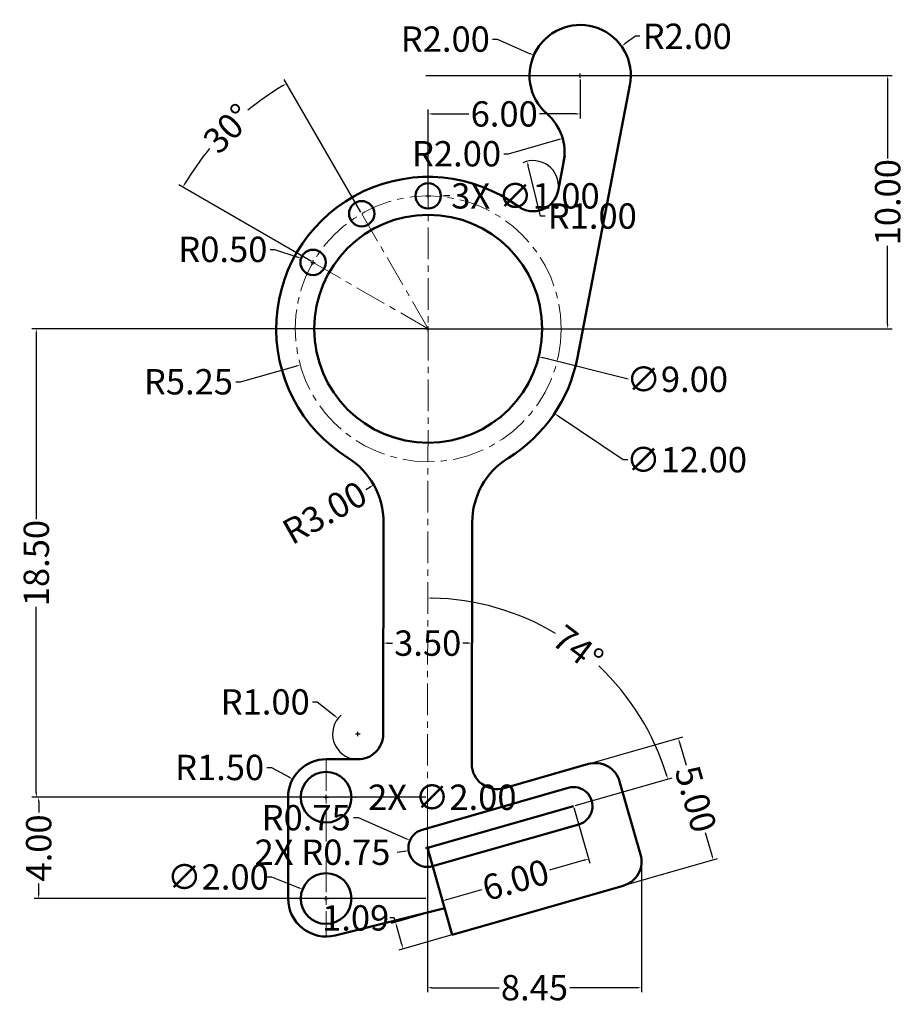
# Model space of a CAD drawing. Units: inches. Extents: x 11.4 to 46.3, y -1.7 to 37.2.
import ezdxf

# ---------------------------------------------------------------- set-up
doc = ezdxf.new("R2010")
doc.units = ezdxf.units.IN
doc.header["$MEASUREMENT"] = 0
doc.linetypes.add('CENTER', pattern=[2, 1.25, -0.25, 0.25, -0.25])
for name, color, linetype, lineweight in [('M-CNTR', 1, 'CENTER', 18), ('M-CONS', 8, 'Continuous', 13), ('M-DIMS', 2, 'Continuous', 25), ('M-OUTL', 7, 'Continuous', 50)]:
    doc.layers.add(name, color=color, linetype=linetype, lineweight=lineweight)
doc.styles.get("Standard").update_dxf_attribs({"font": 'arial.ttf'})
doc.dimstyles.get("Standard").update_dxf_attribs({"dimtxt": 1, "dimasz": 0.18, "dimexe": 0.18, "dimexo": 0.0625, "dimgap": 0.09, "dimtad": 0, "dimtoh": 1, "dimzin": 0, "dimdsep": 46, "dimtxsty": 'Standard', "dimcen": 0.09, "dimadec": 0, "dimazin": 0, "dimtfac": 1, "dimtofl": 0, "dimtmove": 0, "dimatfit": 3, "dimfxl": 1, "dimtolj": 1, "dimtzin": 0, "dimarcsym": 0})

# ---------------------------------------------------------------- blocks, each defined once
blk = doc.blocks.new('*D1')
at = {"layer": 'Defpoints', "color": 0, "transparency": 16777216}
for p in [(32.154, 7.358), (38.748, 4.047), (33.532, 2.552)]:
    blk.add_point(p, dxfattribs=at)
at = {"layer": 'M-DIMS', "color": 0, "lineweight": -2, "transparency": 16777216}
for p, q in [((32.214, 7.375), (37.543, 8.903)), ((37.42, 8.681), (37.677, 7.784)), ((38.699, 4.22), (38.442, 5.117)), ((33.592, 2.569), (38.921, 4.097))]:
    blk.add_line(p, q, dxfattribs=at)
at = {"layer": 'M-DIMS', "color": 0, "transparency": 16777216}
for points in [[(37.449, 8.689), (37.391, 8.672), (37.37, 8.854)], [(38.728, 4.229), (38.67, 4.212), (38.748, 4.047)]]:
    blk.add_solid(points, dxfattribs=at)
at = {"layer": 'M-DIMS', "color": 0, "transparency": 16777216, "insert": (38.059, 6.45), "char_height": 1, "attachment_point": 5, "rotation": 286}
blk.add_mtext('\\A1;5.00', dxfattribs=at)
blk = doc.blocks.new('*D2')
at = {"layer": 'Defpoints', "color": 0, "transparency": 16777216}
for p in [(33.232, 6.172), (27.464, 4.518), (33.83, 4.085)]:
    blk.add_point(p, dxfattribs=at)
at = {"layer": 'M-DIMS', "color": 0, "lineweight": -2, "transparency": 16777216}
for p, q in [((33.249, 6.112), (33.88, 3.912)), ((27.481, 4.458), (28.112, 2.258)), ((33.657, 4.035), (32.282, 3.641)), ((28.236, 2.48), (29.61, 2.875))]:
    blk.add_line(p, q, dxfattribs=at)
at = {"layer": 'M-DIMS', "color": 0, "transparency": 16777216}
for points in [[(33.649, 4.064), (33.665, 4.006), (33.83, 4.085)], [(28.227, 2.509), (28.244, 2.452), (28.063, 2.431)]]:
    blk.add_solid(points, dxfattribs=at)
at = {"layer": 'M-DIMS', "color": 0, "transparency": 16777216, "insert": (30.946, 3.258), "char_height": 1, "attachment_point": 5, "rotation": 16}
blk.add_mtext('\\A1;6.00', dxfattribs=at)
blk = doc.blocks.new('*D3')
at = {"layer": 'Defpoints', "color": 0, "transparency": 16777216}
for p in [(27.495, 25.018), (34.951, 10.945), (27.464, 6.518), (33.232, 6.172), (27.464, 4.518)]:
    blk.add_point(p, dxfattribs=at)
at = {"layer": 'M-DIMS', "color": 0, "lineweight": -2, "transparency": 16777216}
blk.add_line((33.292, 6.189), (37.122, 7.287), dxfattribs=at)
for start, end in [(59.1572, 88.8599), (17.0449, 46.7476)]:
    blk.add_arc((27.461, 4.517), 9.87, start, end, dxfattribs=at)
at = {"layer": 'M-DIMS', "color": 0, "transparency": 16777216}
for points in [[(27.657, 14.355), (27.658, 14.415), (27.477, 14.387)], [(36.926, 7.419), (36.869, 7.402), (36.949, 7.238)]]:
    blk.add_solid(points, dxfattribs=at)
at = {"layer": 'M-DIMS', "color": 0, "transparency": 16777216, "insert": (33.408, 12.395), "char_height": 1, "attachment_point": 5, "rotation": 322.9524}
blk.add_mtext('\\A1;74°', dxfattribs=at)
blk = doc.blocks.new('*D4')
at = {"layer": 'Defpoints', "color": 0, "transparency": 16777216}
for p in [(23.932, 9.637), (24.718, 9.019)]:
    blk.add_point(p, dxfattribs=at)
at = {"layer": 'M-DIMS', "color": 0, "lineweight": -2, "transparency": 16777216}
for p, q in [((22.926, 10.286), (23.106, 10.286)), ((23.106, 10.286), (23.791, 9.748)), ((24.628, 9.019), (24.808, 9.019)), ((24.718, 8.929), (24.718, 9.109))]:
    blk.add_line(p, q, dxfattribs=at)
blk.add_arc((24.718, 9.019), 1, 131.5148, 266.3238, dxfattribs=at)
at = {"layer": 'M-DIMS', "color": 0, "transparency": 16777216}
blk.add_solid([(23.809, 9.772), (23.772, 9.724), (23.932, 9.637)], dxfattribs=at)
at = {"layer": 'M-DIMS', "color": 0, "transparency": 16777216, "insert": (21.061, 10.286), "char_height": 1, "attachment_point": 5}
blk.add_mtext('\\A1;R1.00', dxfattribs=at)
blk = doc.blocks.new('*D5')
at = {"layer": 'Defpoints', "color": 0, "transparency": 16777216}
for p in [(26.777, 4.819), (27.464, 4.518)]:
    blk.add_point(p, dxfattribs=at)
at = {"layer": 'M-DIMS', "color": 0, "lineweight": -2, "transparency": 16777216}
for p, q in [((24.55, 5.715), (24.73, 5.715)), ((24.73, 5.715), (26.612, 4.891)), ((27.374, 4.518), (27.554, 4.518)), ((27.464, 4.428), (27.464, 4.608))]:
    blk.add_line(p, q, dxfattribs=at)
at = {"layer": 'M-DIMS', "color": 0, "transparency": 16777216}
blk.add_solid([(26.624, 4.918), (26.6, 4.863), (26.777, 4.819)], dxfattribs=at)
at = {"layer": 'M-DIMS', "color": 0, "transparency": 16777216, "insert": (22.679, 5.715), "char_height": 1, "attachment_point": 5}
blk.add_mtext('\\A1;R0.75', dxfattribs=at)
blk = doc.blocks.new('*D6')
at = {"layer": 'Defpoints', "color": 0, "transparency": 16777216}
for p in [(22.475, 27.803), (22.948, 27.643)]:
    blk.add_point(p, dxfattribs=at)
at = {"layer": 'M-DIMS', "color": 0, "lineweight": -2, "transparency": 16777216}
for p, q in [((21.254, 28.154), (21.434, 28.154)), ((21.434, 28.154), (22.304, 27.86)), ((22.858, 27.643), (23.038, 27.643)), ((22.948, 27.553), (22.948, 27.733))]:
    blk.add_line(p, q, dxfattribs=at)
at = {"layer": 'M-DIMS', "color": 0, "transparency": 16777216}
blk.add_solid([(22.314, 27.889), (22.294, 27.832), (22.475, 27.803)], dxfattribs=at)
at = {"layer": 'M-DIMS', "color": 0, "transparency": 16777216, "insert": (19.388, 28.154), "char_height": 1, "attachment_point": 5}
blk.add_mtext('\\A1;R0.50', dxfattribs=at)
blk = doc.blocks.new('*D7')
at = {"layer": 'Defpoints', "color": 0, "transparency": 16777216}
for p in [(31.664, 35.821), (33.495, 35.016)]:
    blk.add_point(p, dxfattribs=at)
at = {"layer": 'M-DIMS', "color": 0, "lineweight": -2, "transparency": 16777216}
for p, q in [((30.037, 36.458), (30.217, 36.458)), ((30.217, 36.458), (31.499, 35.894)), ((33.405, 35.016), (33.585, 35.016)), ((33.495, 34.926), (33.495, 35.106))]:
    blk.add_line(p, q, dxfattribs=at)
at = {"layer": 'M-DIMS', "color": 0, "transparency": 16777216}
blk.add_solid([(31.511, 35.921), (31.487, 35.866), (31.664, 35.821)], dxfattribs=at)
at = {"layer": 'M-DIMS', "color": 0, "transparency": 16777216, "insert": (28.171, 36.458), "char_height": 1, "attachment_point": 5}
blk.add_mtext('\\A1;R2.00', dxfattribs=at)
blk = doc.blocks.new('*D8')
at = {"layer": 'Defpoints', "color": 0, "transparency": 16777216}
for p in [(31.402, 31.633), (31.637, 30.661)]:
    blk.add_point(p, dxfattribs=at)
at = {"layer": 'M-DIMS', "color": 0, "lineweight": -2, "transparency": 16777216}
for p, q in [((31.926, 29.47), (31.444, 31.458)), ((32.106, 29.47), (31.926, 29.47))]:
    blk.add_line(p, q, dxfattribs=at)
blk.add_arc((31.637, 30.661), 1, 352.6761, 113.9298, dxfattribs=at)
at = {"layer": 'M-DIMS', "color": 0, "transparency": 16777216}
blk.add_solid([(31.473, 31.465), (31.415, 31.451), (31.402, 31.633)], dxfattribs=at)
at = {"layer": 'M-DIMS', "color": 0, "transparency": 16777216, "insert": (33.971, 29.47), "char_height": 1, "attachment_point": 5}
blk.add_mtext('\\A1;R1.00', dxfattribs=at)
blk = doc.blocks.new('*D9')
at = {"layer": 'Defpoints', "color": 0, "transparency": 16777216}
for p in [(35.124, 36.176), (33.495, 35.016)]:
    blk.add_point(p, dxfattribs=at)
at = {"layer": 'M-DIMS', "color": 0, "lineweight": -2, "transparency": 16777216}
for p, q in [((35.675, 36.569), (35.27, 36.281)), ((35.855, 36.569), (35.675, 36.569)), ((33.405, 35.016), (33.585, 35.016)), ((33.495, 34.926), (33.495, 35.106))]:
    blk.add_line(p, q, dxfattribs=at)
at = {"layer": 'M-DIMS', "color": 0, "transparency": 16777216}
blk.add_solid([(35.253, 36.305), (35.288, 36.256), (35.124, 36.176)], dxfattribs=at)
at = {"layer": 'M-DIMS', "color": 0, "transparency": 16777216, "insert": (37.72, 36.569), "char_height": 1, "attachment_point": 5}
blk.add_mtext('\\A1;R2.00', dxfattribs=at)
blk = doc.blocks.new('*D10')
at = {"layer": 'Defpoints', "color": 0, "transparency": 16777216}
for p in [(32.8, 32.537), (30.875, 31.993)]:
    blk.add_point(p, dxfattribs=at)
at = {"layer": 'M-DIMS', "color": 0, "lineweight": -2, "transparency": 16777216}
for p, q in [((30.658, 31.931), (32.627, 32.488)), ((30.478, 31.931), (30.658, 31.931))]:
    blk.add_line(p, q, dxfattribs=at)
at = {"layer": 'M-DIMS', "color": 0, "transparency": 16777216}
blk.add_solid([(32.619, 32.517), (32.635, 32.459), (32.8, 32.537)], dxfattribs=at)
at = {"layer": 'M-DIMS', "color": 0, "transparency": 16777216, "insert": (28.613, 31.931), "char_height": 1, "attachment_point": 5}
blk.add_mtext('\\A1;R2.00', dxfattribs=at)
blk = doc.blocks.new('*D11')
at = {"layer": 'Defpoints', "color": 0, "transparency": 16777216}
for p in [(33.495, 34.926), (33.495, 33.504), (27.495, 30.268)]:
    blk.add_point(p, dxfattribs=at)
at = {"layer": 'M-DIMS', "color": 0, "lineweight": -2, "transparency": 16777216}
for p, q in [((33.495, 34.863), (33.495, 33.324)), ((27.495, 30.33), (27.495, 33.684)), ((27.675, 33.504), (29.105, 33.504)), ((33.315, 33.504), (31.885, 33.504))]:
    blk.add_line(p, q, dxfattribs=at)
at = {"layer": 'M-DIMS', "color": 0, "transparency": 16777216}
for points in [[(27.675, 33.534), (27.675, 33.474), (27.495, 33.504)], [(33.315, 33.534), (33.315, 33.474), (33.495, 33.504)]]:
    blk.add_solid(points, dxfattribs=at)
at = {"layer": 'M-DIMS', "color": 0, "transparency": 16777216, "insert": (30.495, 33.504), "char_height": 1, "attachment_point": 5}
blk.add_mtext('\\A1;6.00', dxfattribs=at)
blk = doc.blocks.new('*D12')
at = {"layer": 'Defpoints', "color": 0, "transparency": 16777216}
for p in [(25.345, 18.855), (22.732, 17.381)]:
    blk.add_point(p, dxfattribs=at)
at = {"layer": 'M-DIMS', "color": 0, "lineweight": -2, "transparency": 16777216}
blk.add_line((25.032, 18.678), (25.189, 18.767), dxfattribs=at)
at = {"layer": 'M-DIMS', "color": 0, "transparency": 16777216}
blk.add_solid([(25.174, 18.793), (25.203, 18.74), (25.345, 18.855)], dxfattribs=at)
at = {"layer": 'M-DIMS', "color": 0, "transparency": 16777216, "insert": (23.407, 17.762), "char_height": 1, "attachment_point": 5, "rotation": 29.4211}
blk.add_mtext('\\A1;R3.00', dxfattribs=at)
blk = doc.blocks.new('*D13')
at = {"layer": 'Defpoints', "color": 0, "transparency": 16777216}
for p in [(25.725, 13.197), (29.225, 13.191), (29.225, 12.607)]:
    blk.add_point(p, dxfattribs=at)
at = {"layer": 'M-DIMS', "color": 0, "lineweight": -2, "transparency": 16777216}
for p, q in [((25.725, 13.134), (25.725, 12.427)), ((29.225, 13.128), (29.225, 12.427)), ((25.905, 12.607), (26.089, 12.607)), ((29.045, 12.607), (28.862, 12.607))]:
    blk.add_line(p, q, dxfattribs=at)
at = {"layer": 'M-DIMS', "color": 0, "transparency": 16777216}
for points in [[(25.905, 12.637), (25.905, 12.577), (25.725, 12.607)], [(29.045, 12.637), (29.045, 12.577), (29.225, 12.607)]]:
    blk.add_solid(points, dxfattribs=at)
at = {"layer": 'M-DIMS', "color": 0, "transparency": 16777216, "insert": (27.475, 12.607), "char_height": 1, "attachment_point": 5}
blk.add_mtext('\\A1;3.50', dxfattribs=at)
blk = doc.blocks.new('*D14')
at = {"layer": 'Defpoints', "color": 0, "transparency": 16777216}
for p in [(22.147, 7.239), (23.464, 6.521)]:
    blk.add_point(p, dxfattribs=at)
at = {"layer": 'M-DIMS', "color": 0, "lineweight": -2, "transparency": 16777216}
for p, q in [((21.126, 7.697), (21.306, 7.697)), ((21.306, 7.697), (21.989, 7.325)), ((23.464, 6.431), (23.464, 6.611)), ((23.374, 6.521), (23.554, 6.521))]:
    blk.add_line(p, q, dxfattribs=at)
at = {"layer": 'M-DIMS', "color": 0, "transparency": 16777216}
blk.add_solid([(22.003, 7.351), (21.975, 7.298), (22.147, 7.239)], dxfattribs=at)
at = {"layer": 'M-DIMS', "color": 0, "transparency": 16777216, "insert": (19.261, 7.697), "char_height": 1, "attachment_point": 5}
blk.add_mtext('\\A1;R1.50', dxfattribs=at)
blk = doc.blocks.new('*D15')
at = {"layer": 'Defpoints', "color": 0, "transparency": 16777216}
for p in [(22.534, 2.889), (24.394, 2.153)]:
    blk.add_point(p, dxfattribs=at)
at = {"layer": 'M-DIMS', "color": 0, "lineweight": -2, "transparency": 16777216}
for p, q in [((21.126, 3.374), (21.306, 3.374)), ((21.306, 3.374), (22.367, 2.955)), ((23.374, 2.521), (23.554, 2.521)), ((23.464, 2.431), (23.464, 2.611))]:
    blk.add_line(p, q, dxfattribs=at)
at = {"layer": 'M-DIMS', "color": 0, "transparency": 16777216}
blk.add_solid([(22.378, 2.983), (22.356, 2.927), (22.534, 2.889)], dxfattribs=at)
at = {"layer": 'M-DIMS', "color": 0, "transparency": 16777216, "insert": (19.195, 3.374), "char_height": 1, "attachment_point": 5}
blk.add_mtext('\\A1;∅2.00', dxfattribs=at)
blk = doc.blocks.new('*D16')
at = {"layer": 'Defpoints', "color": 0, "transparency": 16777216}
for p in [(27.495, 25.018), (12.025, 6.518), (27.464, 6.518)]:
    blk.add_point(p, dxfattribs=at)
at = {"layer": 'M-DIMS', "color": 0, "lineweight": -2, "transparency": 16777216}
for p, q in [((27.432, 25.018), (11.845, 25.018)), ((12.025, 24.838), (12.025, 17.496)), ((12.025, 6.698), (12.025, 14.039)), ((27.402, 6.518), (11.845, 6.518))]:
    blk.add_line(p, q, dxfattribs=at)
at = {"layer": 'M-DIMS', "color": 0, "transparency": 16777216}
for points in [[(11.995, 24.838), (12.055, 24.838), (12.025, 25.018)], [(11.995, 6.698), (12.055, 6.698), (12.025, 6.518)]]:
    blk.add_solid(points, dxfattribs=at)
at = {"layer": 'M-DIMS', "color": 0, "transparency": 16777216, "insert": (12.025, 15.768), "char_height": 1, "attachment_point": 5, "rotation": 90}
blk.add_mtext('\\A1;18.50', dxfattribs=at)
blk = doc.blocks.new('*D17')
at = {"layer": 'Defpoints', "color": 0, "transparency": 16777216}
for p in [(27.464, 6.518), (12.119, 2.518), (27.464, 2.518)]:
    blk.add_point(p, dxfattribs=at)
at = {"layer": 'M-DIMS', "color": 0, "lineweight": -2, "transparency": 16777216}
for p, q in [((27.402, 6.518), (11.939, 6.518)), ((12.119, 6.338), (12.119, 5.925)), ((12.119, 2.698), (12.119, 3.111)), ((27.402, 2.518), (11.939, 2.518))]:
    blk.add_line(p, q, dxfattribs=at)
at = {"layer": 'M-DIMS', "color": 0, "transparency": 16777216}
for points in [[(12.089, 6.338), (12.149, 6.338), (12.119, 6.518)], [(12.089, 2.698), (12.149, 2.698), (12.119, 2.518)]]:
    blk.add_solid(points, dxfattribs=at)
at = {"layer": 'M-DIMS', "color": 0, "transparency": 16777216, "insert": (12.119, 4.518), "char_height": 1, "attachment_point": 5, "rotation": 90}
blk.add_mtext('\\A1;4.00', dxfattribs=at)
blk = doc.blocks.new('*D18')
at = {"layer": 'Defpoints', "color": 0, "transparency": 16777216}
for p in [(27.339, 35.017), (45.632, 35.017), (27.495, 25.018)]:
    blk.add_point(p, dxfattribs=at)
at = {"layer": 'M-DIMS', "color": 0, "lineweight": -2, "transparency": 16777216}
for p, q in [((27.401, 35.017), (45.812, 35.017)), ((45.632, 34.837), (45.632, 31.746)), ((45.632, 25.198), (45.632, 28.289)), ((27.557, 25.018), (45.812, 25.018))]:
    blk.add_line(p, q, dxfattribs=at)
at = {"layer": 'M-DIMS', "color": 0, "transparency": 16777216}
for points in [[(45.602, 34.837), (45.662, 34.837), (45.632, 35.017)], [(45.602, 25.198), (45.662, 25.198), (45.632, 25.018)]]:
    blk.add_solid(points, dxfattribs=at)
at = {"layer": 'M-DIMS', "color": 0, "transparency": 16777216, "insert": (45.632, 30.017), "char_height": 1, "attachment_point": 5, "rotation": 90}
blk.add_mtext('\\A1;10.00', dxfattribs=at)
blk = doc.blocks.new('*D19')
at = {"layer": 'Defpoints', "color": 0, "transparency": 16777216}
for p in [(27.495, 25.018), (22.442, 23.593)]:
    blk.add_point(p, dxfattribs=at)
at = {"layer": 'M-DIMS', "color": 0, "lineweight": -2, "transparency": 16777216}
for p, q in [((27.405, 25.018), (27.585, 25.018)), ((27.495, 24.928), (27.495, 25.108)), ((20.082, 22.927), (22.269, 23.544)), ((19.902, 22.927), (20.082, 22.927))]:
    blk.add_line(p, q, dxfattribs=at)
at = {"layer": 'M-DIMS', "color": 0, "transparency": 16777216}
blk.add_solid([(22.261, 23.573), (22.277, 23.515), (22.442, 23.593)], dxfattribs=at)
at = {"layer": 'M-DIMS', "color": 0, "transparency": 16777216, "insert": (18.031, 22.927), "char_height": 1, "attachment_point": 5}
blk.add_mtext('\\A1;R5.25', dxfattribs=at)
blk = doc.blocks.new('*D20')
at = {"layer": 'Defpoints', "color": 0, "transparency": 16777216}
for p in [(22.513, 28.362), (32.477, 21.674)]:
    blk.add_point(p, dxfattribs=at)
at = {"layer": 'M-DIMS', "color": 0, "lineweight": -2, "transparency": 16777216}
for p, q in [((27.405, 25.018), (27.585, 25.018)), ((27.495, 24.928), (27.495, 25.108)), ((35.194, 19.849), (32.626, 21.573)), ((35.374, 19.849), (35.194, 19.849))]:
    blk.add_line(p, q, dxfattribs=at)
at = {"layer": 'M-DIMS', "color": 0, "transparency": 16777216}
blk.add_solid([(32.643, 21.598), (32.609, 21.548), (32.477, 21.674)], dxfattribs=at)
at = {"layer": 'M-DIMS', "color": 0, "transparency": 16777216, "insert": (37.693, 19.849), "char_height": 1, "attachment_point": 5}
blk.add_mtext('\\A1;∅12.00', dxfattribs=at)
blk = doc.blocks.new('*D21')
at = {"layer": 'Defpoints', "color": 0, "transparency": 16777216}
for p in [(23.132, 26.118), (31.858, 23.918)]:
    blk.add_point(p, dxfattribs=at)
at = {"layer": 'M-DIMS', "color": 0, "lineweight": -2, "transparency": 16777216}
for p, q in [((27.405, 25.018), (27.585, 25.018)), ((27.495, 24.928), (27.495, 25.108)), ((35.393, 23.026), (32.033, 23.874))]:
    blk.add_line(p, q, dxfattribs=at)
at = {"layer": 'M-DIMS', "color": 0, "transparency": 16777216}
blk.add_solid([(32.04, 23.903), (32.026, 23.845), (31.858, 23.918)], dxfattribs=at)
at = {"layer": 'M-DIMS', "color": 0, "transparency": 16777216, "insert": (37.324, 23.026), "char_height": 1, "attachment_point": 5}
blk.add_mtext('\\A1;∅9.00', dxfattribs=at)
blk = doc.blocks.new('*D22')
at = {"layer": 'Defpoints', "color": 0, "transparency": 16777216}
for p in [(20.305, 33.586), (24.87, 29.564), (22.948, 27.643), (27.495, 25.018), (27.495, 25.018)]:
    blk.add_point(p, dxfattribs=at)
at = {"layer": 'M-DIMS', "color": 0, "lineweight": -2, "transparency": 16777216}
for p, q in [((24.839, 29.619), (21.812, 34.86)), ((22.894, 27.674), (17.653, 30.7))]:
    blk.add_line(p, q, dxfattribs=at)
for start, end in [(120.9221, 129.5076), (140.4924, 149.0779)]:
    blk.add_arc((27.495, 25.018), 11.185, start, end, dxfattribs=at)
at = {"layer": 'M-DIMS', "color": 0, "transparency": 16777216}
for points in [[(21.732, 34.639), (21.762, 34.587), (21.902, 34.704)], [(17.926, 30.75), (17.874, 30.781), (17.808, 30.61)]]:
    blk.add_solid(points, dxfattribs=at)
at = {"layer": 'M-DIMS', "color": 0, "transparency": 16777216, "insert": (19.586, 32.927), "char_height": 1, "attachment_point": 5, "rotation": 45}
blk.add_mtext('\\A1;30°', dxfattribs=at)
blk = doc.blocks.new('*D23')
at = {"layer": 'Defpoints', "color": 0, "transparency": 16777216}
for p in [(27.464, 4.518), (35.915, 4.071), (35.915, -0.999)]:
    blk.add_point(p, dxfattribs=at)
at = {"layer": 'M-DIMS', "color": 0, "lineweight": -2, "transparency": 16777216}
for p, q in [((27.464, 4.455), (27.464, -1.179)), ((35.915, 4.009), (35.915, -1.179)), ((27.644, -0.999), (30.296, -0.999)), ((35.735, -0.999), (33.083, -0.999))]:
    blk.add_line(p, q, dxfattribs=at)
at = {"layer": 'M-DIMS', "color": 0, "transparency": 16777216}
for points in [[(27.644, -0.969), (27.644, -1.029), (27.464, -0.999)], [(35.735, -0.969), (35.735, -1.029), (35.915, -0.999)]]:
    blk.add_solid(points, dxfattribs=at)
at = {"layer": 'M-DIMS', "color": 0, "transparency": 16777216, "insert": (31.689, -0.999), "char_height": 1, "attachment_point": 5}
blk.add_mtext('\\A1;8.45', dxfattribs=at)
blk = doc.blocks.new('*D24')
at = {"layer": 'Defpoints', "color": 0, "transparency": 16777216}
for p in [(28.146, 2.141), (26.204, 1.584), (28.446, 1.093)]:
    blk.add_point(p, dxfattribs=at)
at = {"layer": 'M-DIMS', "color": 0, "lineweight": -2, "transparency": 16777216}
for p, q in [((28.086, 2.124), (26.031, 1.534)), ((26.154, 1.757), (25.974, 1.757)), ((26.204, 1.584), (26.154, 1.757)), ((26.455, 0.709), (26.254, 1.411)), ((28.386, 1.076), (26.331, 0.487))]:
    blk.add_line(p, q, dxfattribs=at)
at = {"layer": 'M-DIMS', "color": 0, "transparency": 16777216}
for points in [[(26.282, 1.419), (26.225, 1.403), (26.204, 1.584)], [(26.484, 0.718), (26.426, 0.701), (26.504, 0.536)]]:
    blk.add_solid(points, dxfattribs=at)
at = {"layer": 'M-DIMS', "color": 0, "transparency": 16777216, "insert": (24.632, 1.757), "char_height": 1, "attachment_point": 5}
blk.add_mtext('\\A1;1.09', dxfattribs=at)
blk = doc.blocks.new('*D25')
at = {"layer": 'Defpoints', "color": 0, "transparency": 16777216}
for p in [(26.995, 30.268), (27.995, 30.268)]:
    blk.add_point(p, dxfattribs=at)
at = {"layer": 'M-DIMS', "color": 0, "lineweight": -2, "transparency": 16777216}
for p, q in [((27.495, 30.178), (27.495, 30.358)), ((27.405, 30.268), (27.585, 30.268)), ((28.355, 30.268), (28.175, 30.268))]:
    blk.add_line(p, q, dxfattribs=at)
at = {"layer": 'M-DIMS', "color": 0, "transparency": 16777216}
blk.add_solid([(28.175, 30.298), (28.175, 30.238), (27.995, 30.268)], dxfattribs=at)
at = {"layer": 'M-DIMS', "color": 0, "transparency": 16777216, "insert": (31.333, 30.268), "char_height": 1, "attachment_point": 5}
blk.add_mtext('\\A1;3X ∅1.00', dxfattribs=at)
blk = doc.blocks.new('*D26')
at = {"layer": 'Defpoints', "color": 0, "transparency": 16777216}
for p in [(22.464, 6.521), (24.464, 6.521)]:
    blk.add_point(p, dxfattribs=at)
at = {"layer": 'M-DIMS', "color": 0, "lineweight": -2, "transparency": 16777216}
for p, q in [((23.464, 6.431), (23.464, 6.611)), ((23.374, 6.521), (23.554, 6.521)), ((25.064, 6.521), (24.644, 6.521))]:
    blk.add_line(p, q, dxfattribs=at)
at = {"layer": 'M-DIMS', "color": 0, "transparency": 16777216}
blk.add_solid([(24.644, 6.551), (24.644, 6.491), (24.464, 6.521)], dxfattribs=at)
at = {"layer": 'M-DIMS', "color": 0, "transparency": 16777216, "insert": (28.052, 6.521), "char_height": 1, "attachment_point": 5}
blk.add_mtext('\\A1;2X ∅2.00', dxfattribs=at)
blk = doc.blocks.new('*D27')
at = {"layer": 'Defpoints', "color": 0, "transparency": 16777216}
for p in [(26.722, 4.413), (27.464, 4.518)]:
    blk.add_point(p, dxfattribs=at)
at = {"layer": 'M-DIMS', "color": 0, "lineweight": -2, "transparency": 16777216}
for p, q in [((26.276, 4.35), (26.543, 4.388)), ((27.374, 4.518), (27.554, 4.518)), ((27.464, 4.428), (27.464, 4.608))]:
    blk.add_line(p, q, dxfattribs=at)
at = {"layer": 'M-DIMS', "color": 0, "transparency": 16777216}
blk.add_solid([(26.539, 4.418), (26.548, 4.358), (26.722, 4.413)], dxfattribs=at)
at = {"layer": 'M-DIMS', "color": 0, "transparency": 16777216, "insert": (23.322, 4.35), "char_height": 1, "attachment_point": 5}
blk.add_mtext('\\A1;2X R0.75', dxfattribs=at)

msp = doc.modelspace()

# ---------------------------------------------------------------- linework, layer by layer
at = {"layer": 'M-CNTR'}
for p, q in [((22.995, 25.018), (31.995, 25.018)), ((23.469, 8.021), (23.464, 1.021))]:
    msp.add_line(p, q, dxfattribs=at)
for points in [[(27.495, 31.018), (27.495, 25.018), (27.464, 6.518)], [(24.87, 29.564), (27.495, 25.018), (22.948, 27.643)], [(27.464, 2.518), (27.464, 6.518), (27.464, 5.518)]]:
    msp.add_lwpolyline(points, dxfattribs=at)
msp.add_circle((27.495, 25.018), 5.25, dxfattribs=at)
at = {"layer": 'M-CONS'}
msp.add_line((23.464, 8.278), (23.464, 8.278), dxfattribs=at)
msp.add_line((23.464, 8.278), (23.464, 8.278), dxfattribs=at)
msp.add_lwpolyline([(23.464, 8.278), (23.464, 8.278)], close=True, dxfattribs=at)
at = {"layer": 'M-OUTL'}
for p, q in [((21.964, 6.521), (21.964, 2.521)), ((23.827, 1.065), (28.146, 2.141))]:
    msp.add_line(p, q, dxfattribs=at)
for points in [[(33.232, 6.172), (27.464, 4.518), (28.446, 1.093), (35.194, 3.028, 0.414214), (35.879, 4.265), (35.052, 7.149, 0.414214), (33.816, 7.834), (30.492, 6.881, -0.499101), (29.216, 7.844), (29.232, 17.37, -0.259291), (30.653, 19.916, 0.209525), (33.387, 23.883), (35.459, 34.637, 1.732051), (32.185, 33.504, -0.267949), (32.839, 31.614)], [(32.888, 31.867), (32.619, 30.471, -0.55076), (31.045, 29.855, 1.038529), (24.32, 19.927, -0.259291), (25.732, 17.376), (25.718, 9.017, -0.414214), (24.717, 8.019), (23.464, 8.021)], [(27.464, 5.268, 1.150368), (27.671, 3.797), (33.438, 5.451, 1), (33.025, 6.893), (27.257, 5.239)]]:
    msp.add_lwpolyline(points, format="xyb", dxfattribs=at)
for centre, radius in [((27.495, 30.268), 0.5), ((24.87, 29.564), 0.5), ((27.495, 25.018), 4.5), ((22.948, 27.643), 0.5), ((23.464, 6.521), 1), ((23.464, 2.521), 1)]:
    msp.add_circle(centre, radius, dxfattribs=at)
for centre, start, end in [((23.464, 6.521), 89.8095, 180), ((23.464, 2.521), 180, 283.985)]:
    msp.add_arc(centre, 1.5, start, end, dxfattribs=at)

# ---------------------------------------------------------------- dimensions: what is measured, and where the dimension line sits
at = {"layer": 'M-DIMS'}
for center, mpoint, picture, middle in [((33.495, 35.016), (31.664, 35.821), '*D7', (28.171, 36.458)), ((33.495, 35.016), (35.124, 36.176), '*D9', (37.72, 36.569)), ((30.875, 31.993), (32.8, 32.537), '*D10', (28.613, 31.931)), ((31.637, 30.661), (31.402, 31.633), '*D8', (33.971, 29.47)), ((22.948, 27.643), (22.475, 27.803), '*D6', (19.388, 28.154)), ((27.495, 25.018), (22.442, 23.593), '*D19', (18.031, 22.927)), ((22.732, 17.381), (25.345, 18.855), '*D12', (23.407, 17.762)), ((24.718, 9.019), (23.932, 9.637), '*D4', (21.061, 10.286)), ((23.464, 6.521), (22.147, 7.239), '*D14', (19.261, 7.697)), ((27.464, 4.518), (26.777, 4.819), '*D5', (22.679, 5.715))]:
    dim = msp.add_radius_dim(center=center, mpoint=mpoint, dimstyle='Standard', override={"dimclrd": 0, "dimclre": 0, "dimclrt": 0}, dxfattribs=at)
    dim.commit()
    dim.dimension.update_dxf_attribs({"geometry": picture, "text_midpoint": middle, "dimtype": 164})
for base, p1, p2, angle, override, picture, middle in [((45.632, 35.017), (27.495, 25.018), (27.339, 35.017), 90, {"dimclrd": 0, "dimclre": 0, "dimclrt": 0}, '*D18', (45.632, 30.017)), ((12.025, 6.518), (27.495, 25.018), (27.464, 6.518), 90, {"dimclrd": 0, "dimclre": 0, "dimclrt": 0}, '*D16', (12.025, 15.768)), ((12.119, 2.518), (27.464, 6.518), (27.464, 2.518), 90, {"dimclrd": 0, "dimclre": 0, "dimclrt": 0}, '*D17', (12.119, 4.518)), ((26.204, 1.584), (28.446, 1.093), (28.146, 2.141), 106, {"dimdec": 2, "dimlfac": 1, "dimrnd": 0, "dimzin": 0, "dimdsep": 46, "dimlunit": 2}, '*D24', (24.632, 1.757))]:
    dim = msp.add_linear_dim(base=base, p1=p1, p2=p2, angle=angle, dimstyle='Standard', override=override, dxfattribs=at)
    dim.commit()
    dim.dimension.update_dxf_attribs({"geometry": picture, "text_midpoint": middle})
for base, line1, line2, picture, middle in [((20.305, 33.586), ((24.87, 29.564), (27.495, 25.018)), ((27.495, 25.018), (22.948, 27.643)), '*D22', (19.586, 32.927)), ((34.951, 10.945), ((33.232, 6.172), (27.464, 4.518)), ((27.495, 25.018), (27.464, 6.518)), '*D3', (33.408, 12.395))]:
    dim = msp.add_angular_dim_2l(base=base, line1=line1, line2=line2, dimstyle='Standard', override={"dimclrd": 0, "dimclre": 0, "dimclrt": 0}, dxfattribs=at)
    dim.commit()
    dim.dimension.update_dxf_attribs({"geometry": picture, "text_midpoint": middle})
for base, p1, p2, override, picture, middle in [((33.495, 33.504), (27.495, 30.268), (33.495, 34.926), {"dimclrd": 0, "dimclre": 0, "dimclrt": 0}, '*D11', (30.495, 33.504)), ((29.225, 12.607), (25.725, 13.197), (29.225, 13.191), {"dimclrd": 0, "dimclre": 0, "dimclrt": 0}, '*D13', (27.475, 12.607)), ((35.915, -0.999), (27.464, 4.518), (35.915, 4.071), {"dimdec": 2, "dimlfac": 1, "dimrnd": 0, "dimzin": 0, "dimdsep": 46, "dimlunit": 2}, '*D23', (31.689, -0.999))]:
    dim = msp.add_linear_dim(base=base, p1=p1, p2=p2, dimstyle='Standard', override=override, dxfattribs=at)
    dim.commit()
    dim.dimension.update_dxf_attribs({"geometry": picture, "text_midpoint": middle})
for p1, p2, text, picture, middle in [((26.995, 30.268), (27.995, 30.268), '3X <>', '*D25', (28.355, 30.268)), ((22.464, 6.521), (24.464, 6.521), '2X <>', '*D26', (25.064, 6.521))]:
    dim = msp.add_diameter_dim_2p(p1=p1, p2=p2, text=text, dimstyle='Standard', override={"dimdec": 2, "dimlfac": 1, "dimrnd": 0, "dimzin": 0, "dimdsep": 46, "dimlunit": 2}, dxfattribs=at)
    dim.commit()
    dim.dimension.update_dxf_attribs({"geometry": picture, "text_midpoint": middle, "dimtype": 163})
for p1, p2, picture, middle in [((22.513, 28.362), (32.477, 21.674), '*D20', (37.693, 19.849)), ((23.132, 26.118), (31.858, 23.918), '*D21', (35.393, 23.026)), ((24.394, 2.153), (22.534, 2.889), '*D15', (19.195, 3.374))]:
    dim = msp.add_diameter_dim_2p(p1=p1, p2=p2, dimstyle='Standard', override={"dimclrd": 0, "dimclre": 0, "dimclrt": 0}, dxfattribs=at)
    dim.commit()
    dim.dimension.update_dxf_attribs({"geometry": picture, "text_midpoint": middle, "dimtype": 163})
for p1, p2, distance, picture, middle in [((32.154, 7.358), (33.532, 2.552), 5.427, '*D1', (38.059, 6.45)), ((27.464, 4.518), (33.232, 6.172), -2.171, '*D2', (30.946, 3.258))]:
    dim = msp.add_aligned_dim(p1=p1, p2=p2, distance=distance, dimstyle='Standard', override={"dimclrd": 0, "dimclre": 0, "dimclrt": 0}, dxfattribs=at)
    dim.commit()
    dim.dimension.update_dxf_attribs({"geometry": picture, "text_midpoint": middle})
dim = msp.add_radius_dim(center=(27.464, 4.518), mpoint=(26.722, 4.413), text='2X <>', dimstyle='Standard', override={"dimdec": 2, "dimlfac": 1, "dimrnd": 0, "dimzin": 0, "dimdsep": 46, "dimlunit": 2}, dxfattribs=at)
dim.commit()
dim.dimension.update_dxf_attribs({"geometry": '*D27', "text_midpoint": (26.276, 4.35), "dimtype": 164})

doc.saveas('drawing.dxf')
